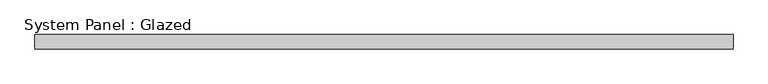
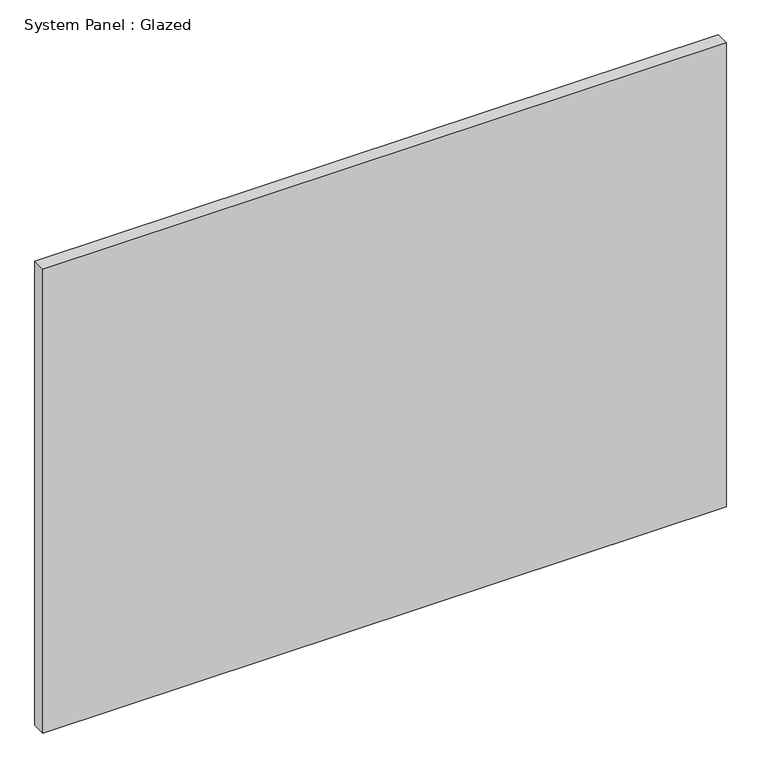
"""IFC4 building model written with IfcOpenShell, lengths in millimetres: plate geometry, System Panel : Glazed."""

from ifc_helpers import new_model, si_unit, origin, origin_with_axes, place, context, project, spatial, polyline, outline, extrude, source, transform, mapped, element, save


def system_panel_glazed_361cf07d(model_context):
    return source(origin(), model_context, "Body", "SweptSolid", [
        extrude(outline(polyline([(625.475, 19.05), (-625.475, 19.05), (-625.475, 44.45), (625.475, 44.45), (625.475, 19.05)])), origin_with_axes(), (0.0, 0.0, 1.0), 897.3037122),
    ])


if __name__ == "__main__":
    model = new_model("IFC4")
    model_context = context("Model", 3, world=origin())
    ifc_project = project(units=[si_unit("LENGTHUNIT", "METRE", prefix="MILLI")], contexts=[model_context])
    site = spatial("IfcSite", under=ifc_project)
    building = spatial("IfcBuilding", under=site)
    placement = place(None, origin())
    system_panel_glazed_shape = system_panel_glazed_361cf07d(model_context)
    element("IfcPlate", 1, ObjectType="System Panel : Glazed", at=placement, inside=building, context=model_context, shape_type="MappedRepresentation", body=[
        mapped(system_panel_glazed_shape, transform((0.0, 0.0, 0.0), x_axis=(1.0, 0.0, 0.0), y_axis=(0.0, 1.0, 0.0), z_axis=(0.0, 0.0, 1.0))),
    ])
    save(model, "model.ifc")

# Revit data of these elements
# Type "System Panel : Glazed"
#   Construction Type Id = "GSP4R"
#   Analytic Construction = "1/8 in Pilkington single glazing"
#   Visual Light Transmittance = 0.9
#   Solar Heat Gain Coefficient = 0.86
#   Heat Transfer Coefficient (U) = 1.18115 BTU/(h·ft²·°F)
#   Define Thermal Properties by = 1
# Element 1 (IfcPlate, "System Panel : Glazed")
#   Materials on its faces: "Glass"
# Materials
#   "Glass": class "Glass", colour RGB 0 128 192, transparency 0.75, Description = "Soda Lime Glass", Cost = 0
